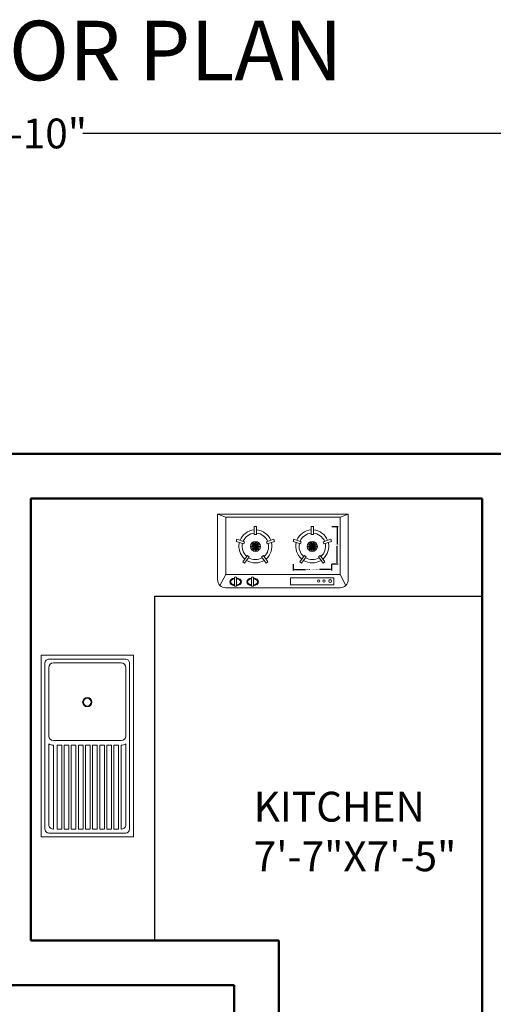
# Model space of a CAD drawing. Units: inches. Extents: x -173 to 545, y -746 to 104.
# Tile 31 of 32: x 263 to 359, y -94 to 104. Entities that reach past the tile are written whole.
import ezdxf

# ---------------------------------------------------------------- set-up
doc = ezdxf.new("R2010")
doc.units = ezdxf.units.IN
doc.header["$MEASUREMENT"] = 0
for name, color, linetype, lineweight in [('A-ANNO-DIMS', 2, 'Continuous', 18), ('A-ANNO-TEXT', 7, 'Continuous', 18), ('A-AREA-IDEN', 7, 'Continuous', 18), ('A-EQPM', 8, 'Continuous', 18), ('A-FLOR-CASE', 9, 'Continuous', 25), ('A-FLOR-FIXT', 8, 'Continuous', 18), ('A-WALL', 7, 'Continuous', 50)]:
    doc.layers.add(name, color=color, linetype=linetype, lineweight=lineweight)
doc.styles.get("Standard").update_dxf_attribs({"font": 'arial.ttf'})
doc.dimstyles.get("Standard").update_dxf_attribs({"dimtxt": 0.18, "dimasz": 0.18, "dimexe": 0.18, "dimexo": 0.0625, "dimgap": 0.09, "dimtad": 0, "dimtih": 1, "dimtoh": 1, "dimdec": 0, "dimzin": 0, "dimdsep": 46, "dimlunit": 3, "dimtxsty": 'Standard', "dimcen": 0.09, "dimadec": 0, "dimazin": 0, "dimtfac": 1, "dimtdec": 0, "dimtofl": 0, "dimtmove": 0, "dimatfit": 3, "dimfxl": 1, "dimtolj": 1, "dimtzin": 0, "dimarcsym": 0})

# ---------------------------------------------------------------- blocks, each defined once
blk = doc.blocks.new('М11 540х1060')
for p, q in [((-1062, 540), (0, 540)), ((-1062, 0), (-1062, 540)), ((0, 540), (0, 0)), ((-1039.5, 45), (-1039.5, 495)), ((-1017, 517.5), (-45, 517.5)), ((-1017, 72), (-1017, 468)), ((-990, 495), (-589.5, 495)), ((-562.5, 72), (-562.5, 468)), ((-543.7, 495), (-64.8, 495)), ((-535.7, 468), (-45, 468)), ((-45, 469.5), (-45, 468)), ((-22.5, 495), (-22.5, 45)), ((-535.7, 453.4), (-45, 453.4)), ((-535.7, 453.4), (-535.7, 426.4)), ((-535.7, 426.4), (-45, 426.4)), ((-535.7, 411.8), (-535.7, 384.8)), ((-535.7, 411.8), (-45, 411.8)), ((-45, 453.4), (-45, 426.4)), ((-45, 411.8), (-45, 384.8)), ((-535.7, 384.8), (-45, 384.8)), ((-535.7, 370.1), (-535.7, 343.1)), ((-535.7, 370.1), (-45, 370.1)), ((-45, 370.1), (-45, 343.1)), ((-535.7, 343.1), (-45, 343.1)), ((-535.7, 328.5), (-535.7, 301.5)), ((-535.7, 328.5), (-45, 328.5)), ((-535.7, 301.5), (-45, 301.5)), ((-45, 328.5), (-45, 301.5)), ((-535.7, 286.9), (-535.7, 259.9)), ((-535.7, 286.9), (-45, 286.9)), ((-535.7, 259.9), (-45, 259.9)), ((-535.7, 245.3), (-535.7, 218.3)), ((-535.7, 245.3), (-45, 245.3)), ((-45, 286.9), (-45, 259.9)), ((-45, 245.3), (-45, 218.3)), ((-535.7, 218.3), (-45, 218.3)), ((-535.7, 203.6), (-535.7, 176.6)), ((-535.7, 203.6), (-45, 203.6)), ((-535.7, 176.6), (-45, 176.6)), ((-45, 203.6), (-45, 176.6)), ((-535.7, 162), (-45, 162)), ((-535.7, 162), (-535.7, 135)), ((-535.7, 135), (-45, 135)), ((-535.7, 120.4), (-45, 120.4)), ((-535.7, 120.4), (-535.7, 93.4)), ((-45, 162), (-45, 135)), ((-45, 120.4), (-45, 93.4)), ((-535.7, 93.4), (-45, 93.4)), ((-535.7, 72), (-45, 72)), ((-535.7, 72), (-535.7, 67.5)), ((-45, 70.5), (-45, 72)), ((0, 0), (-1062, 0)), ((-45, 22.5), (-1017, 22.5)), ((-589.5, 45), (-990, 45)), ((-543.7, 45), (-64.8, 45))]:
    blk.add_line(p, q)
for centre, major_axis, start_param, end_param in [((-1017, 495), (-15.9, 15.9), -0.785398, 0.785398), ((-990, 468), (19.1, 19.1), 0.785398, 2.356194), ((-589.5, 468), (-19.1, 19.1), 3.926991, 5.497787), ((-585.2, 468), (-35, 35), 3.926991, 4.503922), ((-72.3, 468.8), (-19.3, 19.3), 3.899365, 5.250385), ((-45, 495), (15.9, 15.9), 5.497787, 7.068583), ((-787.5, 270), (-19.1, 19.1), 3.926991, 10.210176), ((-787.5, 270), (-15.9, 15.9), 3.926991, 10.210176), ((-990, 72), (-19.1, 19.1), 0.785398, 2.356194), ((-589.5, 72), (19.1, 19.1), 3.926991, 5.497787), ((-585.2, 72), (35, 35), 4.920856, 5.497787), ((-72.3, 71.2), (19.3, 19.3), 4.174393, 5.525413), ((-1017, 45), (15.9, 15.9), 2.356194, 3.926991), ((-45, 45), (-15.9, 15.9), 2.356194, 3.926991)]:
    blk.add_ellipse(centre, major_axis=major_axis, ratio=1, start_param=start_param, end_param=end_param)
blk = doc.blocks.new('*D23')
at = {"layer": 'A-ANNO-DIMS', "color": 0, "lineweight": -2, "transparency": 16777216}
for p, q in [((24.3, 16.7), (24.3, 81.33)), ((501.8, 16.7), (501.8, 81.33)), ((24.48, 81.15), (250.33, 81.15)), ((501.62, 81.15), (275.78, 81.15))]:
    blk.add_line(p, q, dxfattribs=at)
at = {"layer": 'A-ANNO-DIMS', "color": 0, "transparency": 16777216}
for points in [[(24.48, 81.18), (24.48, 81.12), (24.3, 81.15)], [(501.62, 81.18), (501.62, 81.12), (501.8, 81.15)]]:
    blk.add_solid(points, dxfattribs=at)
at = {"layer": 'Defpoints', "color": 0, "transparency": 16777216}
for p in [(501.8, 81.15), (24.3, 16.64), (501.8, 16.64)]:
    blk.add_point(p, dxfattribs=at)
at = {"layer": 'A-ANNO-DIMS', "color": 0, "transparency": 16777216, "insert": (263.05, 81.15), "char_height": 6, "attachment_point": 5}
blk.add_mtext('\\A1;39\'-10"', dxfattribs=at)
blk = doc.blocks.new('HOB-26-BURNER')
for p, q in [((4.1, 7.37), (3.65, 7.37)), ((3.65, 7.37), (3.65, 5.77)), ((4.1, 5.77), (4.1, 7.37)), ((0.14, 4.82), (0, 4.39)), ((0, 4.39), (1.52, 3.9)), ((1.66, 4.32), (0.14, 4.82)), ((1.52, 3.9), (1.66, 4.32)), ((3.87, 3.37), (3.28, 4.19)), ((3.87, 3.37), (3.56, 4.33)), ((3.65, 5.77), (4.1, 5.77)), ((3.87, 3.37), (3.87, 4.38)), ((3.87, 3.37), (4.19, 4.33)), ((3.87, 3.37), (4.47, 4.19)), ((7.61, 4.82), (6.09, 4.32)), ((6.09, 4.32), (6.23, 3.9)), ((6.23, 3.9), (7.75, 4.39)), ((7.75, 4.39), (7.61, 4.82)), ((3.87, 3.37), (2.86, 3.37)), ((3.87, 3.37), (2.91, 3.68)), ((3.87, 3.37), (2.91, 3.06)), ((3.87, 3.37), (3.05, 3.96)), ((3.87, 3.37), (3.05, 2.77)), ((3.87, 3.37), (3.28, 2.55)), ((3.87, 3.37), (3.56, 2.4)), ((3.87, 3.37), (4.7, 3.96)), ((3.87, 3.37), (4.84, 3.68)), ((3.87, 3.37), (3.87, 2.35)), ((3.87, 3.37), (4.19, 2.4)), ((3.87, 3.37), (4.47, 2.55)), ((3.87, 3.37), (4.7, 2.77)), ((3.87, 3.37), (4.84, 3.06)), ((3.87, 3.37), (4.89, 3.37)), ((2.28, 1.56), (1.34, 0.26)), ((1.34, 0.26), (1.7, 0)), ((1.7, 0), (2.64, 1.29)), ((2.64, 1.29), (2.28, 1.56)), ((5.47, 1.56), (5.1, 1.29)), ((5.1, 1.29), (6.04, 0)), ((6.41, 0.26), (5.47, 1.56)), ((6.04, 0), (6.41, 0.26))]:
    blk.add_line(p, q)
blk.add_circle((3.87, 3.37), 1.02)
for radius, start, end in [(3.33, 93.8765, 158.1235), (2.67, 94.8365, 157.1635), (3.33, 21.8765, 86.1235), (2.67, 22.8365, 85.1635), (3.33, 165.8765, 230.1235), (2.67, 166.8365, 229.1635), (2.67, 310.8365, 13.1635), (3.33, 309.8765, 14.1235), (3.33, 237.8765, 302.1235), (2.67, 238.8365, 301.1635)]:
    blk.add_arc((3.87, 3.37), radius, start, end)
blk = doc.blocks.new('COUNTER-L-RETURN')
for p, q in [((66, 69.36), (0, 69.36)), ((66, 0), (66, 69.36))]:
    blk.add_line(p, q)
blk = doc.blocks.new('*D74')
at = {"layer": 'A-ANNO-DIMS', "color": 0, "lineweight": -2, "transparency": 16777216}
for p, q in [((318.18, -5.57), (318.18, -6.85)), ((325.93, -5.57), (325.93, -6.85)), ((318.36, -6.67), (320.65, -6.67)), ((325.75, -6.67), (323.47, -6.67))]:
    blk.add_line(p, q, dxfattribs=at)
at = {"layer": 'A-ANNO-DIMS', "color": 0, "transparency": 16777216}
for points in [[(318.36, -6.64), (318.36, -6.7), (318.18, -6.67)], [(325.75, -6.64), (325.75, -6.7), (325.93, -6.67)]]:
    blk.add_solid(points, dxfattribs=at)
at = {"layer": 'Defpoints', "color": 0, "transparency": 16777216}
for p in [(318.18, -5.51), (325.93, -5.51), (325.93, -6.67)]:
    blk.add_point(p, dxfattribs=at)
at = {"layer": 'A-ANNO-DIMS', "color": 0, "transparency": 16777216, "insert": (322.06, -6.67), "char_height": 0.18, "attachment_point": 5}
blk.add_mtext('\\A1;BURNER 0\'-7 1/2" TYP.', dxfattribs=at)
blk = doc.blocks.new('*D75')
at = {"layer": 'A-ANNO-DIMS', "color": 0, "lineweight": -2, "transparency": 16777216}
for p, q in [((325.99, 1.99), (327.27, 1.99)), ((327.09, 1.81), (327.09, -1.58)), ((327.09, -5.33), (327.09, -1.94)), ((325.99, -5.51), (327.27, -5.51))]:
    blk.add_line(p, q, dxfattribs=at)
at = {"layer": 'A-ANNO-DIMS', "color": 0, "transparency": 16777216}
for points in [[(327.06, 1.81), (327.12, 1.81), (327.09, 1.99)], [(327.06, -5.33), (327.12, -5.33), (327.09, -5.51)]]:
    blk.add_solid(points, dxfattribs=at)
at = {"layer": 'Defpoints', "color": 0, "transparency": 16777216}
for p in [(325.93, 1.99), (327.09, 1.99), (325.93, -5.51)]:
    blk.add_point(p, dxfattribs=at)
at = {"layer": 'A-ANNO-DIMS', "color": 0, "transparency": 16777216, "insert": (327.09, -1.76), "char_height": 0.18, "attachment_point": 5}
blk.add_mtext('\\A1;0\'-7 1/2" TYP.', dxfattribs=at)

msp = doc.modelspace()

# ---------------------------------------------------------------- linework, layer by layer
at = {"layer": 'A-EQPM'}
for p, q in [((302.95, -8.7), (302.95, 4.48)), ((302.95, 4.48), (329.3, 4.48)), ((304.59, 3.85), (302.95, 4.48)), ((327.65, 3.85), (329.3, 4.48)), ((329.3, 4.48), (329.3, -8.7)), ((304.59, -7.68), (304.59, 3.85)), ((304.59, 3.85), (327.65, 3.85)), ((327.65, 3.85), (327.65, -7.68)), ((304.59, -7.68), (303.43, -9.87)), ((327.65, -7.68), (304.59, -7.68)), ((327.65, -7.68), (328.82, -9.87)), ((306.79, -8.23), (306.36, -8.23)), ((306.36, -8.23), (306.36, -10.05)), ((306.79, -10.05), (306.79, -8.23)), ((309.77, -8.23), (309.77, -10.05)), ((310.2, -8.23), (309.77, -8.23)), ((310.2, -10.05), (310.2, -8.23)), ((326.39, -8.37), (317.67, -8.37)), ((317.67, -8.37), (317.67, -9.78)), ((317.67, -9.78), (326.39, -9.78)), ((326.39, -9.78), (326.39, -8.37)), ((327.65, -10.35), (304.59, -10.35)), ((306.36, -10.05), (306.79, -10.05)), ((309.77, -10.05), (310.2, -10.05))]:
    msp.add_line(p, q, dxfattribs=at)
for centre, radius in [((323.33, -9), 0.243), ((324.4, -9), 0.243), ((325.66, -9), 0.292)]:
    msp.add_circle(centre, radius, dxfattribs=at)
for centre, start, end in [((304.59, -8.7), 180, 270), ((327.65, -8.7), 270, 0)]:
    msp.add_arc(centre, 1.65, start, end, dxfattribs=at)
at = {"layer": 'A-EQPM', "extrusion": (0, 0, -1)}
for centre, major_axis, start_param, end_param in [((306.6, -9.15), (1.18, 0), 1.774361, 4.508825), ((306.6, -9.15), (-1.18, 0), 1.73081, 4.552375), ((310.01, -9.15), (1.18, 0), 1.774361, 4.508825), ((310.01, -9.15), (-1.18, 0), 1.73081, 4.552375)]:
    msp.add_ellipse(centre, major_axis=major_axis, ratio=0.671641, start_param=start_param, end_param=end_param, dxfattribs=at)
at = {"layer": 'A-EQPM'}
for points, knots in [([(306.36, -9.76), (306.3, -9.75), (306.25, -9.74), (306.12, -9.7), (306.05, -9.68), (305.93, -9.62), (305.87, -9.59), (305.78, -9.52), (305.74, -9.48), (305.67, -9.4), (305.64, -9.36), (305.6, -9.28), (305.59, -9.24), (305.58, -9.16), (305.58, -9.12), (305.6, -9.04), (305.61, -9), (305.66, -8.92), (305.68, -8.88), (305.76, -8.8), (305.8, -8.76), (305.91, -8.69), (305.96, -8.66), (306.09, -8.61), (306.16, -8.58), (306.27, -8.55), (306.32, -8.55), (306.36, -8.54)], [8.079302, 8.079302, 8.079302, 8.079302, 8.245651, 8.245651, 8.463703, 8.463703, 8.681755, 8.681755, 8.899807, 8.899807, 9.117859, 9.117859, 9.33591, 9.33591, 9.553962, 9.553962, 9.772014, 9.772014, 9.990066, 9.990066, 10.208118, 10.208118, 10.426169, 10.426169, 10.644221, 10.644221, 10.770253, 10.770253, 10.770253, 10.770253]), ([(306.79, -8.53), (306.83, -8.54), (306.87, -8.54), (306.99, -8.57), (307.06, -8.59), (307.19, -8.64), (307.25, -8.67), (307.36, -8.74), (307.41, -8.77), (307.49, -8.85), (307.52, -8.89), (307.57, -8.97), (307.59, -9.01), (307.61, -9.08), (307.61, -9.12), (307.61, -9.15), (307.61, -9.19), (307.61, -9.23), (307.58, -9.31), (307.56, -9.35), (307.5, -9.43), (307.47, -9.47), (307.38, -9.54), (307.33, -9.58), (307.22, -9.64), (307.16, -9.67), (307.02, -9.72), (306.95, -9.74), (306.84, -9.76), (306.82, -9.76), (306.79, -9.76)], [4.889299, 4.889299, 4.889299, 4.889299, 5.015191, 5.015191, 5.233243, 5.233243, 5.451295, 5.451295, 5.669347, 5.669347, 5.887399, 5.887399, 6.10545, 6.10545, 6.283185, 6.283185, 6.283185, 6.501237, 6.501237, 6.719289, 6.719289, 6.937341, 6.937341, 7.155392, 7.155392, 7.373444, 7.373444, 7.591496, 7.591496, 7.677072, 7.677072, 7.677072, 7.677072]), ([(309.77, -9.76), (309.71, -9.75), (309.66, -9.74), (309.53, -9.7), (309.47, -9.68), (309.34, -9.62), (309.29, -9.59), (309.19, -9.52), (309.15, -9.48), (309.08, -9.4), (309.05, -9.36), (309.02, -9.28), (309, -9.24), (308.99, -9.16), (308.99, -9.12), (309.01, -9.04), (309.02, -9), (309.07, -8.92), (309.1, -8.88), (309.17, -8.8), (309.22, -8.76), (309.32, -8.69), (309.38, -8.66), (309.5, -8.61), (309.57, -8.58), (309.69, -8.55), (309.73, -8.55), (309.77, -8.54)], [8.079302, 8.079302, 8.079302, 8.079302, 8.245651, 8.245651, 8.463703, 8.463703, 8.681755, 8.681755, 8.899807, 8.899807, 9.117859, 9.117859, 9.33591, 9.33591, 9.553962, 9.553962, 9.772014, 9.772014, 9.990066, 9.990066, 10.208118, 10.208118, 10.426169, 10.426169, 10.644221, 10.644221, 10.770253, 10.770253, 10.770253, 10.770253]), ([(310.2, -8.53), (310.24, -8.54), (310.29, -8.54), (310.4, -8.57), (310.47, -8.59), (310.6, -8.64), (310.66, -8.67), (310.77, -8.74), (310.82, -8.77), (310.9, -8.85), (310.93, -8.89), (310.98, -8.97), (311, -9.01), (311.02, -9.08), (311.02, -9.12), (311.02, -9.15), (311.02, -9.19), (311.02, -9.23), (310.99, -9.31), (310.97, -9.35), (310.92, -9.43), (310.88, -9.47), (310.79, -9.54), (310.74, -9.58), (310.63, -9.64), (310.57, -9.67), (310.43, -9.72), (310.36, -9.74), (310.26, -9.76), (310.23, -9.76), (310.2, -9.76)], [4.889299, 4.889299, 4.889299, 4.889299, 5.015191, 5.015191, 5.233243, 5.233243, 5.451295, 5.451295, 5.669347, 5.669347, 5.887399, 5.887399, 6.10545, 6.10545, 6.283185, 6.283185, 6.283185, 6.501237, 6.501237, 6.719289, 6.719289, 6.937341, 6.937341, 7.155392, 7.155392, 7.373444, 7.373444, 7.591496, 7.591496, 7.677072, 7.677072, 7.677072, 7.677072])]:
    msp.add_open_spline(points, degree=3, knots=knots, dxfattribs=at)
at = {"layer": 'A-WALL'}
for p, q in [((24.3, 16.64), (501.8, 16.64)), ((265.3, 7.64), (265.3, -81.36)), ((265.3, 7.64), (356.3, 7.64)), ((356.3, 7.64), (356.3, -128.86)), ((265.3, -81.36), (315.3, -81.36)), ((315.3, -81.36), (315.3, -128.86)), ((260.8, -90.36), (265.3, -90.36)), ((265.3, -90.36), (306.3, -90.36)), ((306.3, -90.36), (306.3, -128.86))]:
    msp.add_line(p, q, dxfattribs=at)

# ---------------------------------------------------------------- block references
at = {"layer": 'A-EQPM'}
for p in [(306.71, -5.38), (318.18, -5.38)]:
    msp.add_blockref('HOB-26-BURNER', p, dxfattribs=at)
at = {"layer": 'A-FLOR-CASE', "extrusion": (0, 0, -1), "zscale": -1}
msp.add_blockref('COUNTER-L-RETURN', (-356.3, -81.36), dxfattribs=at)
at = {"layer": 'A-FLOR-FIXT', "xscale": 0.0344518369672997, "yscale": 0.0344518369672997, "zscale": 0.0344518369672997, "rotation": 270}
msp.add_blockref('М11 540х1060', (267.38, -60.51), dxfattribs=at)

# ---------------------------------------------------------------- texts
at = {"layer": 'A-ANNO-TEXT', "insert": (183.35, 103.85), "char_height": 12, "attachment_point": 1}
msp.add_mtext('FIRST FLOOR PLAN', dxfattribs=at)
at = {"layer": 'A-AREA-IDEN', "insert": (310.24, -51.43), "char_height": 6, "attachment_point": 1}
msp.add_mtext('KITCHEN\\P7\'-7"X7\'-5"', dxfattribs=at)

# ---------------------------------------------------------------- dimensions: what is measured, and where the dimension line sits
at = {"layer": 'A-ANNO-DIMS'}
dim = msp.add_linear_dim(base=(501.80136521, 81.15311648), p1=(24.30136521, 16.63801408), p2=(501.80136521, 16.63801408), dimstyle='Standard', override={"dimtxt": 6, "dimclrd": 0, "dimclre": 0, "dimclrt": 0}, dxfattribs=at)
dim.commit()
dim.dimension.update_dxf_attribs({"geometry": '*D23', "text_midpoint": (263.05136521, 81.15311648)})
dim = msp.add_linear_dim(base=(327.09, 1.99), p1=(325.93, -5.51), p2=(325.93, 1.99), angle=90, text='<> TYP.', dimstyle='Standard', override={"dimdec": 1, "dimlfac": 1, "dimrnd": 0, "dimzin": 1, "dimdsep": 46, "dimlunit": 4, "dimfrac": 2}, dxfattribs=at)
dim.commit()
dim.dimension.update_dxf_attribs({"geometry": '*D75', "text_midpoint": (327.09, -1.76)})
dim = msp.add_linear_dim(base=(325.9317, -6.6688), p1=(318.1827, -5.5064), p2=(325.9317, -5.5064), text='BURNER <> TYP.', dimstyle='Standard', override={"dimdec": 1, "dimlfac": 1, "dimrnd": 0, "dimzin": 1, "dimdsep": 46, "dimlunit": 4, "dimfrac": 2}, dxfattribs=at)
dim.commit()
dim.dimension.update_dxf_attribs({"geometry": '*D74', "text_midpoint": (322.0572, -6.6688)})

doc.saveas('drawing.dxf')
